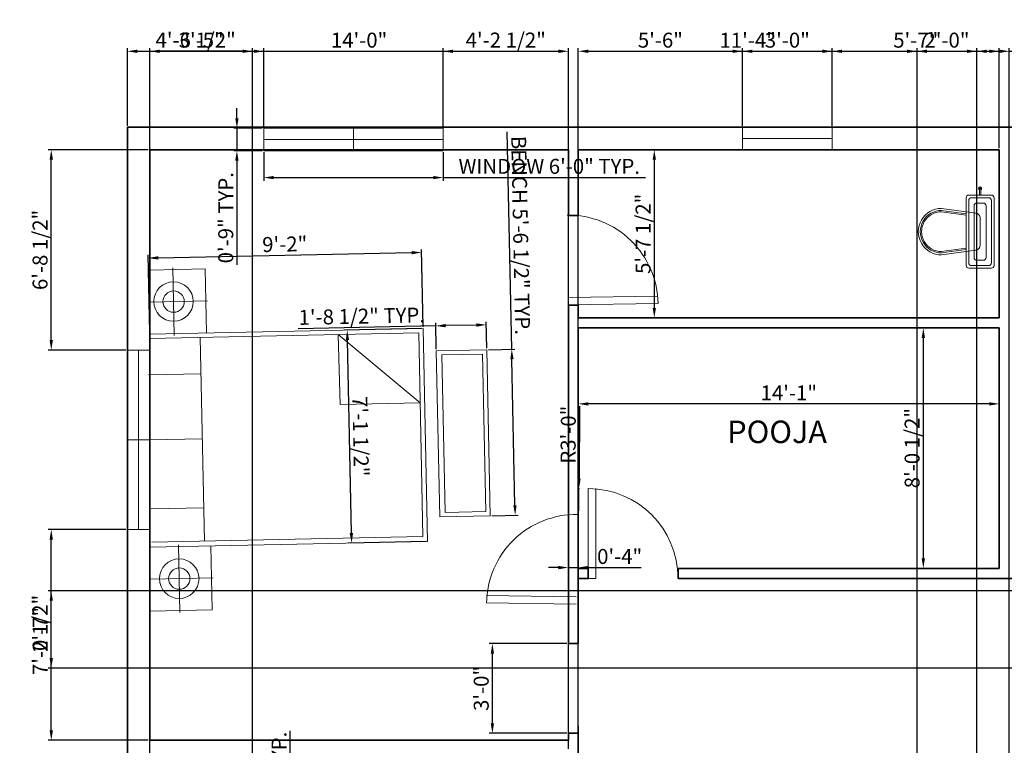
# Model space of a CAD drawing. Units: inches. Extents: x 1973 to 2661, y 1730 to 2412.
# Tile 3 of 5: x 1973 to 2368, y 2117 to 2409. Entities that reach past the tile are written whole.
import ezdxf

# ---------------------------------------------------------------- set-up
doc = ezdxf.new("R2010")
doc.units = ezdxf.units.IN
doc.linetypes.add('ACAD_ISO03W100', pattern=[30, 12, -18])
for name, color, linetype, lineweight in [('A-ANNO-DIMS', 2, 'Continuous', 18), ('A-AREA-IDEN', 7, 'Continuous', 25), ('A-DOOR', 3, 'Continuous', 18), ('A-FLOR-FIXT', 9, 'Continuous', 18), ('A-FLOR-FIXT-HIDN', 9, 'ACAD_ISO03W100', 13), ('A-FURN', 8, 'Continuous', 18), ('A-GLAZ', 4, 'Continuous', 18), ('A-WALL', 7, 'Continuous', 35)]:
    doc.layers.add(name, color=color, linetype=linetype, lineweight=lineweight)
doc.styles.get("Standard").update_dxf_attribs({"font": 'arial.ttf'})
doc.dimstyles.new('ISO-25', dxfattribs={"dimtxt": 6, "dimasz": 4, "dimexe": 1.25, "dimexo": 0.625, "dimtad": 1, "dimdec": 0, "dimrnd": 6, "dimlunit": 3, "dimtxsty": 'Standard', "dimcen": 2.5, "dimadec": 0, "dimazin": 0, "dimtfac": 1, "dimtdec": 0, "dimtmove": 0, "dimatfit": 3, "dimfxl": 1, "dimarcsym": 0})

# ---------------------------------------------------------------- blocks, each defined once
blk = doc.blocks.new('DOOR-36-SWING')
for p, q in [((0, 0), (0, 36)), ((0, 36), (0, 0)), ((3, 0), (3, 36)), ((0, 0), (3, 0))]:
    blk.add_line(p, q)
blk.add_arc((0, 0), 36, 0, 90)
blk = doc.blocks.new('WIN-72-TWO-LIGHT')
for p, q in [((0, 72), (9, 72)), ((0, 0), (0, 72)), ((4.5, 72), (4.5, 36)), ((9, 72), (9, 0)), ((4.5, 36), (0, 36)), ((0, 36), (9, 36)), ((4.5, 36), (4.5, 0)), ((9, 0), (0, 0))]:
    blk.add_line(p, q)
blk = doc.blocks.new('WC-TANK-PLAN')
for p, q in [((9.95, 11.2), (8.6, 21.07)), ((10.75, 11.2), (9.39, 21.19)), ((11.29, 11.2), (9.92, 21.26)), ((25.95, 21.26), (24.57, 11.2)), ((26.48, 21.19), (25.11, 11.2)), ((27.27, 21.07), (25.92, 11.2)), ((3.27, 1.07), (3.27, 10.13)), ((31.53, 11.2), (4.33, 11.2)), ((4.33, 2.13), (4.33, 9.07)), ((30.47, 10.13), (5.4, 10.13)), ((28.33, 8), (7.53, 8)), ((31.53, 2.13), (31.53, 9.07)), ((32.6, 1.07), (32.6, 10.13)), ((0.94, 5.6), (0.22, 5.6)), ((0.6, 5.33), (0.6, 5.87)), ((3.27, 5.87), (0.6, 5.87)), ((3.27, 5.33), (0.6, 5.33)), ((6.47, 4.27), (6.47, 6.93)), ((29.4, 4.27), (29.4, 6.93)), ((30.47, 1.07), (5.4, 1.07)), ((28.33, 3.2), (7.53, 3.2)), ((31.53, 0), (4.33, 0))]:
    blk.add_line(p, q)
for centre, radius, start, end in [((17.93, 21.07), 9.33, 0, 180), ((17.93, 21.07), 8.53, 0, 180), ((17.93, 21.07), 8, 0, 180), ((4.33, 10.13), 1.07, 90, 180), ((5.4, 9.07), 1.07, 90, 180), ((7.53, 6.93), 1.07, 90, 180), ((28.33, 6.93), 1.07, 0, 90), ((30.47, 9.07), 1.07, 0, 90), ((31.53, 10.13), 1.07, 0, 90), ((0.6, 5.6), 0.599, 26.4407, 333.5593), ((7.53, 4.27), 1.07, 180, 270), ((28.33, 4.27), 1.07, 270, 0), ((4.33, 1.07), 1.07, 180, 270), ((5.4, 2.13), 1.07, 180, 270), ((30.47, 2.13), 1.07, 270, 0), ((31.53, 1.07), 1.07, 270, 0)]:
    blk.add_arc(centre, radius, start, end)
blk = doc.blocks.new('BENCH-BED-END')
for p, q in [((0, 20.3), (0, 0)), ((66.64, 20.3), (0, 20.3)), ((66.64, 0), (66.64, 20.3)), ((1.73, 1.73), (1.73, 18.14)), ((1.73, 18.14), (64.92, 18.14)), ((64.92, 18.14), (64.92, 1.73)), ((64.92, 1.73), (1.73, 1.73)), ((0, 0), (66.64, 0))]:
    blk.add_line(p, q)
blk = doc.blocks.new('*D14')
at = {"layer": 'A-ANNO-DIMS', "color": 0, "lineweight": -2, "transparency": 16777216}
for p, q in [((2070.79, 2355.34), (2070.79, 2343.92)), ((2142.79, 2355.34), (2142.79, 2343.92)), ((2074.79, 2345.17), (2138.79, 2345.17)), ((2142.79, 2345.17), (2223.97, 2345.17))]:
    blk.add_line(p, q, dxfattribs=at)
at = {"layer": 'A-ANNO-DIMS', "color": 0, "transparency": 16777216}
for points in [[(2074.79, 2345.83), (2074.79, 2344.5), (2070.79, 2345.17)], [(2138.79, 2345.83), (2138.79, 2344.5), (2142.79, 2345.17)]]:
    blk.add_solid(points, dxfattribs=at)
at = {"layer": 'Defpoints', "color": 0, "transparency": 16777216}
for p in [(2070.79, 2355.97), (2142.79, 2355.97), (2142.79, 2345.17)]:
    blk.add_point(p, dxfattribs=at)
at = {"layer": 'A-ANNO-DIMS', "color": 0, "transparency": 16777216, "insert": (2185.38, 2348.9), "char_height": 6, "attachment_point": 5}
blk.add_mtext('WINDOW 6\'-0" TYP.', dxfattribs=at)
blk = doc.blocks.new('*D15')
at = {"layer": 'A-ANNO-DIMS', "color": 0, "lineweight": -2, "transparency": 16777216}
for p, q in [((2059.99, 2368.97), (2059.99, 2372.97)), ((2070.17, 2364.97), (2058.74, 2364.97)), ((2059.99, 2364.97), (2059.99, 2355.97)), ((2070.17, 2355.97), (2058.74, 2355.97)), ((2059.99, 2351.97), (2059.99, 2310.14))]:
    blk.add_line(p, q, dxfattribs=at)
at = {"layer": 'A-ANNO-DIMS', "color": 0, "transparency": 16777216}
for points in [[(2059.33, 2368.97), (2060.66, 2368.97), (2059.99, 2364.97)], [(2059.33, 2351.97), (2060.66, 2351.97), (2059.99, 2355.97)]]:
    blk.add_solid(points, dxfattribs=at)
at = {"layer": 'Defpoints', "color": 0, "transparency": 16777216}
for p in [(2070.79, 2364.97), (2059.99, 2355.97), (2070.79, 2355.97)]:
    blk.add_point(p, dxfattribs=at)
at = {"layer": 'A-ANNO-DIMS', "color": 0, "transparency": 16777216, "insert": (2056.3, 2329.06), "char_height": 6, "attachment_point": 5, "rotation": 90}
blk.add_mtext('0\'-9" TYP.', dxfattribs=at)
blk = doc.blocks.new('*D21')
at = {"layer": 'A-ANNO-DIMS', "color": 0, "lineweight": -2, "transparency": 16777216}
for p, q in [((2081.33, 2081.84), (2081.33, 2123.1)), ((2084.06, 2081.84), (2080.08, 2081.84)), ((2081.33, 2066.85), (2081.33, 2077.84)), ((2084.06, 2062.85), (2080.08, 2062.85))]:
    blk.add_line(p, q, dxfattribs=at)
at = {"layer": 'A-ANNO-DIMS', "color": 0, "transparency": 16777216}
for points in [[(2080.67, 2077.84), (2082, 2077.84), (2081.33, 2081.84)], [(2080.67, 2066.85), (2082, 2066.85), (2081.33, 2062.85)]]:
    blk.add_solid(points, dxfattribs=at)
at = {"layer": 'Defpoints', "color": 0, "transparency": 16777216}
for p in [(2081.33, 2081.84), (2084.68, 2081.84), (2084.68, 2062.85)]:
    blk.add_point(p, dxfattribs=at)
at = {"layer": 'A-ANNO-DIMS', "color": 0, "transparency": 16777216, "insert": (2077.7, 2104.47), "char_height": 6, "attachment_point": 5, "rotation": 90}
blk.add_mtext('1\'-7" TYP.', dxfattribs=at)
blk = doc.blocks.new('*D24')
at = {"layer": 'A-ANNO-DIMS', "color": 0, "lineweight": -2, "transparency": 16777216}
for p, q in [((2170.33, 2276.29), (2168.54, 2363.48)), ((2160.96, 2276.1), (2171.58, 2276.32)), ((2171.62, 2213.66), (2170.41, 2272.29)), ((2162.33, 2209.47), (2172.95, 2209.69))]:
    blk.add_line(p, q, dxfattribs=at)
at = {"layer": 'A-ANNO-DIMS', "color": 0, "transparency": 16777216}
for points in [[(2171.08, 2272.31), (2169.75, 2272.28), (2170.33, 2276.29)], [(2172.28, 2213.68), (2170.95, 2213.65), (2171.7, 2209.66)]]:
    blk.add_solid(points, dxfattribs=at)
at = {"layer": 'Defpoints', "color": 0, "transparency": 16777216}
for p in [(2160.34, 2276.09), (2170.33, 2276.29), (2161.7, 2209.46)]:
    blk.add_point(p, dxfattribs=at)
at = {"layer": 'A-ANNO-DIMS', "color": 0, "transparency": 16777216, "insert": (2173.12, 2321.96), "char_height": 6, "attachment_point": 5, "rotation": 271.1773}
blk.add_mtext('BENCH 5\'-6 1/2" TYP.', dxfattribs=at)
blk = doc.blocks.new('*D25')
at = {"layer": 'A-ANNO-DIMS', "color": 0, "lineweight": -2, "transparency": 16777216}
for p, q in [((2139.83, 2285.66), (2084.6, 2284.53)), ((2140.02, 2276.29), (2139.81, 2286.91)), ((2156.13, 2286), (2143.83, 2285.75)), ((2160.32, 2276.71), (2160.1, 2287.33))]:
    blk.add_line(p, q, dxfattribs=at)
at = {"layer": 'A-ANNO-DIMS', "color": 0, "transparency": 16777216}
for points in [[(2143.82, 2286.41), (2143.84, 2285.08), (2139.83, 2285.66)], [(2156.12, 2286.67), (2156.14, 2285.33), (2160.13, 2286.08)]]:
    blk.add_solid(points, dxfattribs=at)
at = {"layer": 'Defpoints', "color": 0, "transparency": 16777216}
for p in [(2139.83, 2285.66), (2140.04, 2275.67), (2160.34, 2276.09)]:
    blk.add_point(p, dxfattribs=at)
at = {"layer": 'A-ANNO-DIMS', "color": 0, "transparency": 16777216, "insert": (2110.14, 2288.78), "char_height": 6, "attachment_point": 5, "rotation": 1.1773}
blk.add_mtext('1\'-8 1/2" TYP.', dxfattribs=at)
blk = doc.blocks.new('*D32')
at = {"layer": 'A-ANNO-DIMS', "color": 0, "lineweight": -2, "transparency": 16777216}
for p, q in [((2016.04, 2365.98), (2016.04, 2397.1)), ((2020.04, 2395.85), (2066.79, 2395.85)), ((2070.79, 2365.59), (2070.79, 2397.1))]:
    blk.add_line(p, q, dxfattribs=at)
at = {"layer": 'A-ANNO-DIMS', "color": 0, "transparency": 16777216}
for points in [[(2020.04, 2396.52), (2020.04, 2395.18), (2016.04, 2395.85)], [(2066.79, 2396.52), (2066.79, 2395.18), (2070.79, 2395.85)]]:
    blk.add_solid(points, dxfattribs=at)
at = {"layer": 'Defpoints', "color": 0, "transparency": 16777216}
for p in [(2070.79, 2395.85), (2016.04, 2365.35), (2070.79, 2364.97)]:
    blk.add_point(p, dxfattribs=at)
at = {"layer": 'A-ANNO-DIMS', "color": 0, "transparency": 16777216, "insert": (2043.42, 2399.58), "char_height": 6, "attachment_point": 5}
blk.add_mtext('4\'-6 1/2"', dxfattribs=at)
blk = doc.blocks.new('*D33')
at = {"layer": 'A-ANNO-DIMS', "color": 0, "lineweight": -2, "transparency": 16777216}
for p, q in [((2142.79, 2365.59), (2142.79, 2397.1)), ((2146.79, 2395.85), (2189.04, 2395.85)), ((2193.04, 2356.98), (2193.04, 2397.1))]:
    blk.add_line(p, q, dxfattribs=at)
at = {"layer": 'A-ANNO-DIMS', "color": 0, "transparency": 16777216}
for points in [[(2146.79, 2396.52), (2146.79, 2395.18), (2142.79, 2395.85)], [(2189.04, 2396.52), (2189.04, 2395.18), (2193.04, 2395.85)]]:
    blk.add_solid(points, dxfattribs=at)
at = {"layer": 'Defpoints', "color": 0, "transparency": 16777216}
for p in [(2193.04, 2395.85), (2142.79, 2364.97), (2193.04, 2356.35)]:
    blk.add_point(p, dxfattribs=at)
at = {"layer": 'A-ANNO-DIMS', "color": 0, "transparency": 16777216, "insert": (2167.92, 2399.58), "char_height": 6, "attachment_point": 5}
blk.add_mtext('4\'-2 1/2"', dxfattribs=at)
blk = doc.blocks.new('*D34')
at = {"layer": 'A-ANNO-DIMS', "color": 0, "lineweight": -2, "transparency": 16777216}
for p, q in [((2197.04, 2356.98), (2197.04, 2397.1)), ((2201.04, 2395.85), (2258.95, 2395.85)), ((2262.95, 2365.95), (2262.95, 2397.1))]:
    blk.add_line(p, q, dxfattribs=at)
at = {"layer": 'A-ANNO-DIMS', "color": 0, "transparency": 16777216}
for points in [[(2201.04, 2396.52), (2201.04, 2395.18), (2197.04, 2395.85)], [(2258.95, 2396.52), (2258.95, 2395.18), (2262.95, 2395.85)]]:
    blk.add_solid(points, dxfattribs=at)
at = {"layer": 'Defpoints', "color": 0, "transparency": 16777216}
for p in [(2262.95, 2395.85), (2262.95, 2365.32), (2197.04, 2356.35)]:
    blk.add_point(p, dxfattribs=at)
at = {"layer": 'A-ANNO-DIMS', "color": 0, "transparency": 16777216, "insert": (2229.99, 2399.54), "char_height": 6, "attachment_point": 5}
blk.add_mtext('5\'-6"', dxfattribs=at)
blk = doc.blocks.new('*D35')
at = {"layer": 'A-ANNO-DIMS', "color": 0, "lineweight": -2, "transparency": 16777216}
for p, q in [((2262.95, 2365.95), (2262.95, 2397.1)), ((2266.95, 2395.85), (2294.95, 2395.85)), ((2298.95, 2365.95), (2298.95, 2397.1))]:
    blk.add_line(p, q, dxfattribs=at)
at = {"layer": 'A-ANNO-DIMS', "color": 0, "transparency": 16777216}
for points in [[(2266.95, 2396.52), (2266.95, 2395.18), (2262.95, 2395.85)], [(2294.95, 2396.52), (2294.95, 2395.18), (2298.95, 2395.85)]]:
    blk.add_solid(points, dxfattribs=at)
at = {"layer": 'Defpoints', "color": 0, "transparency": 16777216}
for p in [(2298.95, 2395.85), (2262.95, 2365.32), (2298.95, 2365.32)]:
    blk.add_point(p, dxfattribs=at)
at = {"layer": 'A-ANNO-DIMS', "color": 0, "transparency": 16777216, "insert": (2280.95, 2399.54), "char_height": 6, "attachment_point": 5}
blk.add_mtext('3\'-0"', dxfattribs=at)
blk = doc.blocks.new('*D36')
at = {"layer": 'A-ANNO-DIMS', "color": 0, "lineweight": -2, "transparency": 16777216}
for p, q in [((2298.95, 2365.95), (2298.95, 2397.1)), ((2302.95, 2395.85), (2362.04, 2395.85)), ((2366.04, 2356.98), (2366.04, 2397.1))]:
    blk.add_line(p, q, dxfattribs=at)
at = {"layer": 'A-ANNO-DIMS', "color": 0, "transparency": 16777216}
for points in [[(2302.95, 2396.52), (2302.95, 2395.18), (2298.95, 2395.85)], [(2362.04, 2396.52), (2362.04, 2395.18), (2366.04, 2395.85)]]:
    blk.add_solid(points, dxfattribs=at)
at = {"layer": 'Defpoints', "color": 0, "transparency": 16777216}
for p in [(2366.04, 2395.85), (2298.95, 2365.32), (2366.04, 2356.35)]:
    blk.add_point(p, dxfattribs=at)
at = {"layer": 'A-ANNO-DIMS', "color": 0, "transparency": 16777216, "insert": (2332.49, 2399.53), "char_height": 6, "attachment_point": 5}
blk.add_mtext('5\'-7"', dxfattribs=at)
blk = doc.blocks.new('*D44')
at = {"layer": 'A-ANNO-DIMS', "color": 0, "lineweight": -2, "transparency": 16777216}
for p, q in [((2015.35, 2203.93), (1984.22, 2203.93)), ((1985.47, 2123.35), (1985.47, 2199.93)), ((2024.42, 2119.35), (1984.22, 2119.35))]:
    blk.add_line(p, q, dxfattribs=at)
at = {"layer": 'A-ANNO-DIMS', "color": 0, "transparency": 16777216}
for points in [[(1984.81, 2199.93), (1986.14, 2199.93), (1985.47, 2203.93)], [(1984.81, 2123.35), (1986.14, 2123.35), (1985.47, 2119.35)]]:
    blk.add_solid(points, dxfattribs=at)
at = {"layer": 'Defpoints', "color": 0, "transparency": 16777216}
for p in [(1985.47, 2203.93), (2015.97, 2203.93), (2025.04, 2119.35)]:
    blk.add_point(p, dxfattribs=at)
at = {"layer": 'A-ANNO-DIMS', "color": 0, "transparency": 16777216, "insert": (1981.75, 2161.64), "char_height": 6, "attachment_point": 5, "rotation": 90}
blk.add_mtext('7\'-0 1/2"', dxfattribs=at)
blk = doc.blocks.new('*D45')
at = {"layer": 'A-ANNO-DIMS', "color": 0, "lineweight": -2, "transparency": 16777216}
for p, q in [((2024.42, 2356.35), (1984.22, 2356.35)), ((1985.47, 2279.93), (1985.47, 2352.35)), ((2015.35, 2275.93), (1984.22, 2275.93))]:
    blk.add_line(p, q, dxfattribs=at)
at = {"layer": 'A-ANNO-DIMS', "color": 0, "transparency": 16777216}
for points in [[(1984.81, 2352.35), (1986.14, 2352.35), (1985.47, 2356.35)], [(1984.81, 2279.93), (1986.14, 2279.93), (1985.47, 2275.93)]]:
    blk.add_solid(points, dxfattribs=at)
at = {"layer": 'Defpoints', "color": 0, "transparency": 16777216}
for p in [(1985.47, 2356.35), (2025.04, 2356.35), (2015.97, 2275.93)]:
    blk.add_point(p, dxfattribs=at)
at = {"layer": 'A-ANNO-DIMS', "color": 0, "transparency": 16777216, "insert": (1981.75, 2316.14), "char_height": 6, "attachment_point": 5, "rotation": 90}
blk.add_mtext('6\'-8 1/2"', dxfattribs=at)
blk = doc.blocks.new('*D46')
at = {"layer": 'A-ANNO-DIMS', "color": 0, "lineweight": -2, "transparency": 16777216}
for p, q in [((2025.04, 2115.98), (2025.04, 2397.1)), ((2029.04, 2395.85), (2189.04, 2395.85)), ((2193.04, 2115.98), (2193.04, 2397.1))]:
    blk.add_line(p, q, dxfattribs=at)
at = {"layer": 'A-ANNO-DIMS', "color": 0, "transparency": 16777216}
for points in [[(2029.04, 2396.52), (2029.04, 2395.18), (2025.04, 2395.85)], [(2189.04, 2396.52), (2189.04, 2395.18), (2193.04, 2395.85)]]:
    blk.add_solid(points, dxfattribs=at)
at = {"layer": 'Defpoints', "color": 0, "transparency": 16777216}
for p in [(2193.04, 2395.85), (2025.04, 2115.35), (2193.04, 2115.35)]:
    blk.add_point(p, dxfattribs=at)
at = {"layer": 'A-ANNO-DIMS', "color": 0, "transparency": 16777216, "insert": (2109.04, 2399.54), "char_height": 6, "attachment_point": 5}
blk.add_mtext('14\'-0"', dxfattribs=at)
blk = doc.blocks.new('*D47')
at = {"layer": 'A-ANNO-DIMS', "color": 0, "lineweight": -2, "transparency": 16777216}
for p, q in [((2197.67, 2356.35), (2228.79, 2356.35)), ((2227.54, 2352.35), (2227.54, 2292.85)), ((2197.67, 2288.85), (2228.79, 2288.85))]:
    blk.add_line(p, q, dxfattribs=at)
at = {"layer": 'A-ANNO-DIMS', "color": 0, "transparency": 16777216}
for points in [[(2226.88, 2352.35), (2228.21, 2352.35), (2227.54, 2356.35)], [(2226.88, 2292.85), (2228.21, 2292.85), (2227.54, 2288.85)]]:
    blk.add_solid(points, dxfattribs=at)
at = {"layer": 'Defpoints', "color": 0, "transparency": 16777216}
for p in [(2197.04, 2356.35), (2197.04, 2288.85), (2227.54, 2288.85)]:
    blk.add_point(p, dxfattribs=at)
at = {"layer": 'A-ANNO-DIMS', "color": 0, "transparency": 16777216, "insert": (2223.81, 2322.6), "char_height": 6, "attachment_point": 5, "rotation": 90}
blk.add_mtext('5\'-7 1/2"', dxfattribs=at)
blk = doc.blocks.new('*D48')
at = {"layer": 'A-ANNO-DIMS', "color": 0, "lineweight": -2, "transparency": 16777216}
for p, q in [((2365.42, 2284.85), (2334.29, 2284.85)), ((2335.54, 2192.35), (2335.54, 2280.85)), ((2365.42, 2188.35), (2334.29, 2188.35))]:
    blk.add_line(p, q, dxfattribs=at)
at = {"layer": 'A-ANNO-DIMS', "color": 0, "transparency": 16777216}
for points in [[(2334.88, 2280.85), (2336.21, 2280.85), (2335.54, 2284.85)], [(2334.88, 2192.35), (2336.21, 2192.35), (2335.54, 2188.35)]]:
    blk.add_solid(points, dxfattribs=at)
at = {"layer": 'Defpoints', "color": 0, "transparency": 16777216}
for p in [(2335.54, 2284.85), (2366.04, 2284.85), (2366.04, 2188.35)]:
    blk.add_point(p, dxfattribs=at)
at = {"layer": 'A-ANNO-DIMS', "color": 0, "transparency": 16777216, "insert": (2331.81, 2236.6), "char_height": 6, "attachment_point": 5, "rotation": 90}
blk.add_mtext('8\'-0 1/2"', dxfattribs=at)
blk = doc.blocks.new('*D49')
at = {"layer": 'A-ANNO-DIMS', "color": 0, "lineweight": -2, "transparency": 16777216}
for p, q in [((2197.04, 2284.23), (2197.04, 2253.1)), ((2366.04, 2284.23), (2366.04, 2253.1)), ((2362.04, 2254.35), (2201.04, 2254.35))]:
    blk.add_line(p, q, dxfattribs=at)
at = {"layer": 'A-ANNO-DIMS', "color": 0, "transparency": 16777216}
for points in [[(2201.04, 2255.02), (2201.04, 2253.68), (2197.04, 2254.35)], [(2362.04, 2255.02), (2362.04, 2253.68), (2366.04, 2254.35)]]:
    blk.add_solid(points, dxfattribs=at)
at = {"layer": 'Defpoints', "color": 0, "transparency": 16777216}
for p in [(2197.04, 2284.85), (2366.04, 2284.85), (2197.04, 2254.35)]:
    blk.add_point(p, dxfattribs=at)
at = {"layer": 'A-ANNO-DIMS', "color": 0, "transparency": 16777216, "insert": (2281.54, 2257.99), "char_height": 6, "attachment_point": 5}
blk.add_mtext('14\'-1"', dxfattribs=at)
blk = doc.blocks.new('*D54')
at = {"layer": 'A-ANNO-DIMS', "color": 0, "lineweight": -2, "transparency": 16777216}
for p, q in [((2197.04, 1834.98), (2197.04, 2397.1)), ((2201.04, 2395.85), (2329.03, 2395.85)), ((2333.03, 1834.87), (2333.03, 2397.1))]:
    blk.add_line(p, q, dxfattribs=at)
at = {"layer": 'A-ANNO-DIMS', "color": 0, "transparency": 16777216}
for points in [[(2201.04, 2396.52), (2201.04, 2395.18), (2197.04, 2395.85)], [(2329.03, 2396.52), (2329.03, 2395.18), (2333.03, 2395.85)]]:
    blk.add_solid(points, dxfattribs=at)
at = {"layer": 'Defpoints', "color": 0, "transparency": 16777216}
for p in [(2333.03, 2395.85), (2197.04, 1834.35), (2333.03, 1834.25)]:
    blk.add_point(p, dxfattribs=at)
at = {"layer": 'A-ANNO-DIMS', "color": 0, "transparency": 16777216, "insert": (2265.03, 2399.49), "char_height": 6, "attachment_point": 5}
blk.add_mtext('11\'-4"', dxfattribs=at)
blk = doc.blocks.new('*D61')
at = {"layer": 'A-ANNO-DIMS', "color": 0, "lineweight": -2, "transparency": 16777216}
for p, q in [((2606.42, 2179.35), (1984.22, 2179.35)), ((1985.47, 2152.35), (1985.47, 2175.35)), ((2606.42, 2148.35), (1984.22, 2148.35))]:
    blk.add_line(p, q, dxfattribs=at)
at = {"layer": 'A-ANNO-DIMS', "color": 0, "transparency": 16777216}
for points in [[(1984.81, 2175.35), (1986.14, 2175.35), (1985.47, 2179.35)], [(1984.81, 2152.35), (1986.14, 2152.35), (1985.47, 2148.35)]]:
    blk.add_solid(points, dxfattribs=at)
at = {"layer": 'Defpoints', "color": 0, "transparency": 16777216}
for p in [(1985.47, 2179.35), (2607.04, 2179.35), (2607.04, 2148.35)]:
    blk.add_point(p, dxfattribs=at)
at = {"layer": 'A-ANNO-DIMS', "color": 0, "transparency": 16777216, "insert": (1981.84, 2163.85), "char_height": 6, "attachment_point": 5, "rotation": 90}
blk.add_mtext('2\'-7"', dxfattribs=at)
blk = doc.blocks.new('*D66')
at = {"layer": 'A-ANNO-DIMS', "color": 0, "lineweight": -2, "transparency": 16777216}
for p, q in [((2333.03, 1843.98), (2333.03, 2397.1)), ((2337.03, 2395.85), (2353.02, 2395.85)), ((2357.02, 1843.98), (2357.02, 2397.1))]:
    blk.add_line(p, q, dxfattribs=at)
at = {"layer": 'A-ANNO-DIMS', "color": 0, "transparency": 16777216}
for points in [[(2337.03, 2396.52), (2337.03, 2395.18), (2333.03, 2395.85)], [(2353.02, 2396.52), (2353.02, 2395.18), (2357.02, 2395.85)]]:
    blk.add_solid(points, dxfattribs=at)
at = {"layer": 'Defpoints', "color": 0, "transparency": 16777216}
for p in [(2357.02, 2395.85), (2333.03, 1843.35), (2357.02, 1843.35)]:
    blk.add_point(p, dxfattribs=at)
at = {"layer": 'A-ANNO-DIMS', "color": 0, "transparency": 16777216, "insert": (2345.02, 2399.54), "char_height": 6, "attachment_point": 5}
blk.add_mtext('2\'-0"', dxfattribs=at)
blk = doc.blocks.new('*D69')
at = {"layer": 'A-ANNO-DIMS', "color": 0, "lineweight": -2, "transparency": 16777216}
for p, q in [((2357.02, 1843.98), (2357.02, 2397.1)), ((2361.02, 2395.85), (2366.04, 2395.85)), ((2370.04, 1843.98), (2370.04, 2397.1)), ((2370.04, 2395.85), (2390.68, 2395.85))]:
    blk.add_line(p, q, dxfattribs=at)
at = {"layer": 'A-ANNO-DIMS', "color": 0, "transparency": 16777216}
for points in [[(2361.02, 2396.52), (2361.02, 2395.18), (2357.02, 2395.85)], [(2366.04, 2396.52), (2366.04, 2395.18), (2370.04, 2395.85)]]:
    blk.add_solid(points, dxfattribs=at)
at = {"layer": 'Defpoints', "color": 0, "transparency": 16777216}
for p in [(2370.04, 2395.85), (2357.02, 1843.35), (2370.04, 1843.35)]:
    blk.add_point(p, dxfattribs=at)
at = {"layer": 'A-ANNO-DIMS', "color": 0, "transparency": 16777216, "insert": (2382.36, 2399.49), "char_height": 6, "attachment_point": 5}
blk.add_mtext('1\'-1"', dxfattribs=at)
blk = doc.blocks.new('*D72')
at = {"layer": 'A-ANNO-DIMS', "color": 0, "lineweight": -2, "transparency": 16777216}
for p, q in [((2025.04, 1930.6), (2025.04, 2397.1)), ((2062.26, 2395.85), (2029.04, 2395.85)), ((2066.26, 1930.6), (2066.26, 2397.1))]:
    blk.add_line(p, q, dxfattribs=at)
at = {"layer": 'A-ANNO-DIMS', "color": 0, "transparency": 16777216}
for points in [[(2029.04, 2396.52), (2029.04, 2395.18), (2025.04, 2395.85)], [(2062.26, 2396.52), (2062.26, 2395.18), (2066.26, 2395.85)]]:
    blk.add_solid(points, dxfattribs=at)
at = {"layer": 'Defpoints', "color": 0, "transparency": 16777216}
for p in [(2025.04, 2395.85), (2025.04, 1929.97), (2066.26, 1929.97)]:
    blk.add_point(p, dxfattribs=at)
at = {"layer": 'A-ANNO-DIMS', "color": 0, "transparency": 16777216, "insert": (2045.65, 2399.54), "char_height": 6, "attachment_point": 5}
blk.add_mtext('3\'-5"', dxfattribs=at)
blk = doc.blocks.new('*D76')
at = {"layer": 'A-ANNO-DIMS', "color": 0, "lineweight": -2, "transparency": 16777216}
for p, q in [((2192.42, 2158.17), (2161.29, 2158.17)), ((2162.54, 2126.17), (2162.54, 2154.17)), ((2192.42, 2122.17), (2161.29, 2122.17))]:
    blk.add_line(p, q, dxfattribs=at)
at = {"layer": 'A-ANNO-DIMS', "color": 0, "transparency": 16777216}
for points in [[(2161.88, 2154.17), (2163.21, 2154.17), (2162.54, 2158.17)], [(2161.88, 2126.17), (2163.21, 2126.17), (2162.54, 2122.17)]]:
    blk.add_solid(points, dxfattribs=at)
at = {"layer": 'Defpoints', "color": 0, "transparency": 16777216}
for p in [(2162.54, 2158.17), (2193.04, 2158.17), (2193.04, 2122.17)]:
    blk.add_point(p, dxfattribs=at)
at = {"layer": 'A-ANNO-DIMS', "color": 0, "transparency": 16777216, "insert": (2158.85, 2140.17), "char_height": 6, "attachment_point": 5, "rotation": 90}
blk.add_mtext('3\'-0"', dxfattribs=at)
blk = doc.blocks.new('*D77')
at = {"layer": 'A-ANNO-DIMS', "color": 0, "lineweight": -2, "transparency": 16777216}
for p, q in [((2193.04, 2158.79), (2193.04, 2189.92)), ((2197.04, 2158.79), (2197.04, 2189.92)), ((2189.04, 2188.67), (2185.04, 2188.67)), ((2193.04, 2188.67), (2197.04, 2188.67)), ((2201.04, 2188.67), (2222.24, 2188.67))]:
    blk.add_line(p, q, dxfattribs=at)
at = {"layer": 'A-ANNO-DIMS', "color": 0, "transparency": 16777216}
for points in [[(2189.04, 2189.34), (2189.04, 2188), (2193.04, 2188.67)], [(2201.04, 2189.34), (2201.04, 2188), (2197.04, 2188.67)]]:
    blk.add_solid(points, dxfattribs=at)
at = {"layer": 'Defpoints', "color": 0, "transparency": 16777216}
for p in [(2197.04, 2188.67), (2193.04, 2158.17), (2197.04, 2158.17)]:
    blk.add_point(p, dxfattribs=at)
at = {"layer": 'A-ANNO-DIMS', "color": 0, "transparency": 16777216, "insert": (2213.64, 2192.36), "char_height": 6, "attachment_point": 5}
blk.add_mtext('0\'-4"', dxfattribs=at)
blk = doc.blocks.new('*D80')
at = {"layer": 'A-ANNO-DIMS', "color": 0, "lineweight": -2, "transparency": 16777216}
for p, q in [((2134.76, 2285.25), (2134.12, 2316.37)), ((2025.03, 2283), (2024.39, 2314.12)), ((2028.41, 2312.95), (2130.15, 2315.04))]:
    blk.add_line(p, q, dxfattribs=at)
at = {"layer": 'A-ANNO-DIMS', "color": 0, "transparency": 16777216}
for points in [[(2028.4, 2313.61), (2028.43, 2312.28), (2024.42, 2312.87)], [(2130.14, 2315.71), (2130.17, 2314.37), (2134.15, 2315.12)]]:
    blk.add_solid(points, dxfattribs=at)
at = {"layer": 'Defpoints', "color": 0, "transparency": 16777216}
for p in [(2134.15, 2315.12), (2134.78, 2284.63), (2025.04, 2282.37)]:
    blk.add_point(p, dxfattribs=at)
at = {"layer": 'A-ANNO-DIMS', "color": 0, "transparency": 16777216, "insert": (2079.21, 2317.68), "char_height": 6, "attachment_point": 5, "rotation": 1.1773}
blk.add_mtext('9\'-2"', dxfattribs=at)
blk = doc.blocks.new('*D81')
at = {"layer": 'A-ANNO-DIMS', "color": 0, "lineweight": -2, "transparency": 16777216}
for p, q in [((2134.15, 2284.61), (2103.03, 2283.97)), ((2105.96, 2202.49), (2104.37, 2280)), ((2135.91, 2199.11), (2104.79, 2198.47))]:
    blk.add_line(p, q, dxfattribs=at)
at = {"layer": 'A-ANNO-DIMS', "color": 0, "transparency": 16777216}
for points in [[(2105.03, 2280.01), (2103.7, 2279.99), (2104.28, 2284)], [(2106.63, 2202.51), (2105.29, 2202.48), (2106.04, 2198.49)]]:
    blk.add_solid(points, dxfattribs=at)
at = {"layer": 'Defpoints', "color": 0, "transparency": 16777216}
for p in [(2134.78, 2284.63), (2104.28, 2284), (2136.53, 2199.12)]:
    blk.add_point(p, dxfattribs=at)
at = {"layer": 'A-ANNO-DIMS', "color": 0, "transparency": 16777216, "insert": (2108.89, 2241.32), "char_height": 6, "attachment_point": 5, "rotation": 271.1773}
blk.add_mtext('7\'-1 1/2"', dxfattribs=at)
blk = doc.blocks.new('*D83')
at = {"layer": 'A-ANNO-DIMS', "color": 0, "lineweight": -2, "transparency": 16777216}
for p, q in [((2197.54, 2253.42), (2197.33, 2224.35)), ((2197.04, 2184.35), (2197.3, 2220.35))]:
    blk.add_line(p, q, dxfattribs=at)
at = {"layer": 'A-ANNO-DIMS', "color": 0, "transparency": 16777216}
blk.add_solid([(2196.67, 2224.36), (2198, 2224.35), (2197.3, 2220.35)], dxfattribs=at)
at = {"layer": 'Defpoints', "color": 0, "transparency": 16777216}
for p in [(2197.3, 2220.35), (2197.04, 2184.35)]:
    blk.add_point(p, dxfattribs=at)
at = {"layer": 'A-ANNO-DIMS', "color": 0, "transparency": 16777216, "insert": (2193.77, 2241.98), "char_height": 6, "attachment_point": 5, "rotation": 89.5833}
blk.add_mtext('R3\'-0"', dxfattribs=at)

msp = doc.modelspace()

# ---------------------------------------------------------------- linework, layer by layer
at = {"layer": 'A-DOOR'}
for p, q in [((2197.04, 2187.35), (2197.09, 2187.35)), ((2197.09, 2187.35), (2197.04, 2187.35)), ((2197.09, 2187.35), (2197.04, 2187.35)), ((2197.04, 2187.35), (2197.09, 2187.35)), ((2160.2, 2174.49), (2196.19, 2173.97)), ((2196.19, 2173.97), (2160.2, 2174.49)), ((2160.24, 2177.49), (2196.23, 2176.97))]:
    msp.add_line(p, q, dxfattribs=at)
for centre, end in [((2197.04, 2184.35), 90), ((2197.04, 2184.35), 90), ((2197.04, 2184.35), 90), ((2197.04, 2184.35), 90), ((2196.19, 2173.97), 179.1676)]:
    msp.add_arc(centre, 36, 89.1676, end, dxfattribs=at)
at = {"layer": 'A-FLOR-FIXT-HIDN'}
msp.add_lwpolyline([(2352.72, 2331.46), (2356.5, 2330.95, -0.371763), (2358.32, 2328.83), (2358.32, 2318.12, -0.371763), (2356.5, 2316), (2352.72, 2315.49)], format="xyb", dxfattribs=at)
at = {"layer": 'A-FURN'}
for p, q in [((2025.04, 2308.04), (2047.26, 2308.49)), ((2034.85, 2281.85, -15.39), (2034.29, 2308.99, -15.39)), ((2047.26, 2308.49), (2047.79, 2282.84)), ((2025.04, 2295.22, -15.39), (2048.14, 2295.7, -15.39)), ((2134.78, 2284.63), (2025.04, 2282.37)), ((2136.53, 2199.12), (2134.78, 2284.63)), ((2132.98, 2282.86), (2025.04, 2280.65)), ((2046.98, 2199.33), (2045.3, 2281.06)), ((2101.49, 2254.15), (2100.58, 2282.2)), ((2100.58, 2282.2), (2133.55, 2254.81)), ((2134.66, 2201.13), (2132.98, 2282.86)), ((2024.44, 2265.95), (2045.6, 2266.39)), ((2133.55, 2254.81), (2101.49, 2254.15)), ((2024.97, 2239.93), (2046.14, 2240.37)), ((2024.99, 2228.83), (2025.04, 2226.21)), ((2025.54, 2212.27), (2046.71, 2212.71)), ((2025.04, 2196.83), (2136.53, 2199.12)), ((2025.82, 2198.89), (2134.66, 2201.13)), ((2037.13, 2170.65, -15.39), (2036.57, 2197.79, -15.39)), ((2050.07, 2171.68), (2049.54, 2197.33)), ((2025.04, 2183.98, -15.39), (2050.42, 2184.5, -15.39)), ((2025.04, 2171.16), (2050.07, 2171.68))]:
    msp.add_line(p, q, dxfattribs=at)
for centre, radius in [((2034.57, 2295.42, -15.39), 7.93), ((2034.57, 2295.42, -15.39), 4.28), ((2036.85, 2184.22, -15.39), 7.93), ((2036.85, 2184.22, -15.39), 4.28)]:
    msp.add_circle(centre, radius, dxfattribs=at)
at = {"layer": 'A-GLAZ'}
for p, q in [((2262.95, 2365.32), (2298.95, 2365.32)), ((2262.95, 2356.32), (2262.95, 2365.32)), ((2262.95, 2365.32), (2262.95, 2360.82)), ((2279.57, 2365.32), (2298.95, 2365.32)), ((2298.95, 2365.32), (2298.95, 2356.32)), ((2262.95, 2360.82), (2298.95, 2360.82)), ((2298.95, 2360.82), (2279.57, 2360.82)), ((2298.95, 2356.32), (2262.95, 2356.32)), ((2279.57, 2356.35), (2279.57, 2356.32)), ((2279.57, 2356.32), (2298.95, 2356.32))]:
    msp.add_line(p, q, dxfattribs=at)
at = {"layer": 'A-WALL'}
for p, q in [((2016.04, 1765.35), (2016.04, 2365.35)), ((2016.04, 2365.35), (2616.04, 2365.35)), ((2025.04, 2119.35), (2025.04, 2356.35)), ((2025.04, 2356.35), (2193.04, 2356.35)), ((2193.04, 2356.35), (2193.04, 2329.91)), ((2193.04, 2329.91), (2193.04, 2356.35)), ((2197.04, 2329.91), (2197.04, 2356.35)), ((2197.04, 2356.35), (2366.04, 2356.35)), ((2366.04, 2356.35), (2366.04, 2288.85)), ((2193.04, 2329.91), (2197.04, 2329.91)), ((2197.04, 2293.91), (2193.04, 2293.91)), ((2193.04, 2293.91), (2193.04, 2158.17)), ((2197.04, 2288.85), (2197.04, 2293.91)), ((2366.04, 2288.85), (2197.04, 2288.85)), ((2197.04, 2188.35), (2197.04, 2284.85)), ((2197.04, 2284.85), (2366.04, 2284.85)), ((2366.04, 2284.85), (2366.04, 2188.35)), ((2197.04, 2184.35), (2197.04, 2188.35)), ((2197.04, 2188.35), (2201.06, 2188.35)), ((2197.04, 2187.35), (2197.04, 2184.35)), ((2197.04, 2184.35), (2197.04, 2187.35)), ((2197.04, 2187.35), (2197.04, 2184.35)), ((2201.06, 2188.35), (2201.06, 2184.35)), ((2366.04, 2188.35), (2237.06, 2188.35)), ((2237.06, 2188.35), (2237.06, 2184.35)), ((2197.04, 2158.17), (2197.04, 2184.35)), ((2197.04, 2184.35), (2201.06, 2184.35)), ((2201.06, 2184.35), (2197.04, 2184.35)), ((2237.06, 2184.35), (2375.94, 2184.35)), ((2193.04, 2158.17), (2197.04, 2158.17)), ((2197.04, 2112.1), (2197.04, 2125.17)), ((2197.04, 2125.17), (2197.04, 2122.17)), ((2193.04, 2119.35), (2025.04, 2119.35)), ((2193.04, 2122.23), (2193.04, 2119.35)), ((2197.04, 2122.17), (2193.04, 2122.17)), ((2193.04, 2122.17), (2193.04, 2119.35))]:
    msp.add_line(p, q, dxfattribs=at)

# ---------------------------------------------------------------- block references
at = {"layer": 'A-DOOR', "extrusion": (0, 0, -1), "zscale": -1, "rotation": 89.16759712053707}
msp.add_blockref('DOOR-36-SWING', (-2193.07, 2294.09), dxfattribs=at)
at = {"layer": 'A-DOOR'}
msp.add_blockref('DOOR-36-SWING', (2201.06, 2184.35), dxfattribs=at)
at = {"layer": 'A-FLOR-FIXT', "extrusion": (0, 0, -1), "zscale": -1, "rotation": 269.999999999998}
msp.add_blockref('WC-TANK-PLAN', (-2363.92, 2341.41), dxfattribs=at)
at = {"layer": 'A-FURN', "rotation": 91.17731989174982}
msp.add_blockref('BENCH-BED-END', (2161.7, 2209.46), dxfattribs=at)
at = {"layer": 'A-GLAZ', "rotation": 269.9999999999997}
msp.add_blockref('WIN-72-TWO-LIGHT', (2070.79, 2364.97), dxfattribs=at)
at = {"layer": 'A-GLAZ'}
msp.add_blockref('WIN-72-TWO-LIGHT', (2015.97, 2203.93), dxfattribs=at)

# ---------------------------------------------------------------- texts
at = {"layer": 'A-AREA-IDEN', "insert": (2256.83, 2247.64), "char_height": 9, "attachment_point": 1}
msp.add_mtext_dynamic_manual_height_columns('POOJA', width=6.3229, gutter_width=12.5, heights=[0], dxfattribs=at)

# ---------------------------------------------------------------- dimensions: what is measured, and where the dimension line sits
at = {"layer": 'A-ANNO-DIMS'}
for base, p1, p2, picture, middle in [((2070.792, 2395.8513), (2016.0422, 2365.3513), (2070.792, 2364.9675), '*D32', (2043.4171, 2399.5786)), ((2193.0422, 2395.8513), (2142.792, 2364.9675), (2193.0422, 2356.3513), '*D33', (2167.9171, 2399.5786)), ((2193.04, 2395.85), (2025.04, 2115.35), (2193.04, 2115.35), '*D46', (2109.04, 2399.54)), ((2025.04, 2395.85), (2066.26, 1929.97), (2025.04, 1929.97), '*D72', (2045.65, 2399.54)), ((2262.95, 2395.85), (2197.04, 2356.35), (2262.95, 2365.32), '*D34', (2229.99, 2399.54)), ((2333.03, 2395.85), (2197.04, 1834.35), (2333.03, 1834.25), '*D54', (2265.03, 2399.49)), ((2298.95, 2395.85), (2262.95, 2365.32), (2298.95, 2365.32), '*D35', (2280.95, 2399.54)), ((2366.04, 2395.85), (2298.95, 2365.32), (2366.04, 2356.35), '*D36', (2332.49, 2399.53)), ((2357.02, 2395.85), (2333.03, 1843.35), (2357.02, 1843.35), '*D66', (2345.02, 2399.54)), ((2370.04, 2395.85), (2357.02, 1843.35), (2370.04, 1843.35), '*D69', (2382.36, 2399.49)), ((2197.04, 2188.67), (2193.04, 2158.17), (2197.04, 2158.17), '*D77', (2213.64, 2192.36))]:
    dim = msp.add_linear_dim(base=base, p1=p1, p2=p2, dimstyle='ISO-25', override={"dimdec": 1, "dimlfac": 1, "dimrnd": 0, "dimzin": 1, "dimdsep": 46, "dimlunit": 4, "dimfrac": 2}, dxfattribs=at)
    dim.commit()
    dim.dimension.update_dxf_attribs({"geometry": picture, "text_midpoint": middle})
for base, p1, p2, angle, text, picture, middle in [((2059.99, 2355.97), (2070.79, 2364.97), (2070.79, 2355.97), 270, '<> TYP.', '*D15', (2056.3, 2329.06)), ((2170.33, 2276.29), (2161.7, 2209.46), (2160.34, 2276.09), 91.1773, 'BENCH <> TYP.', '*D24', (2173.12, 2321.96)), ((2139.83, 2285.66), (2160.34, 2276.09), (2140.04, 2275.67), 181.1773, '<> TYP.', '*D25', (2110.14, 2288.78)), ((2081.33, 2081.84), (2084.68, 2062.85), (2084.68, 2081.84), 90, '<> TYP.', '*D21', (2077.7, 2104.47))]:
    dim = msp.add_linear_dim(base=base, p1=p1, p2=p2, angle=angle, text=text, dimstyle='ISO-25', override={"dimdec": 1, "dimlfac": 1, "dimrnd": 0, "dimzin": 1, "dimdsep": 46, "dimlunit": 4, "dimfrac": 2}, dxfattribs=at)
    dim.commit()
    dim.dimension.update_dxf_attribs({"geometry": picture, "text_midpoint": middle})
dim = msp.add_linear_dim(base=(2142.79, 2345.17), p1=(2070.79, 2355.97), p2=(2142.79, 2355.97), text='WINDOW <> TYP.', dimstyle='ISO-25', override={"dimdec": 1, "dimlfac": 1, "dimrnd": 0, "dimzin": 1, "dimdsep": 46, "dimlunit": 4, "dimfrac": 2}, dxfattribs=at)
dim.commit()
dim.dimension.update_dxf_attribs({"geometry": '*D14', "text_midpoint": (2185.38, 2348.9)})
for base, p1, p2, angle, picture, middle in [((1985.47, 2356.35), (2015.97, 2275.93), (2025.04, 2356.35), 90, '*D45', (1981.75, 2316.14)), ((2227.54, 2288.85), (2197.04, 2356.35), (2197.04, 2288.85), 270, '*D47', (2223.81, 2322.6)), ((2134.15, 2315.12), (2025.04, 2282.37), (2134.78, 2284.63), 1.1773, '*D80', (2079.21, 2317.68)), ((2104.28, 2284), (2136.53, 2199.12), (2134.78, 2284.63), 91.1773, '*D81', (2108.89, 2241.32)), ((2197.04, 2254.35), (2366.04, 2284.85), (2197.04, 2284.85), 180, '*D49', (2281.54, 2257.99)), ((2335.54, 2284.85), (2366.04, 2188.35), (2366.04, 2284.85), 90, '*D48', (2331.81, 2236.6)), ((1985.47, 2203.93), (2025.04, 2119.35), (2015.97, 2203.93), 90, '*D44', (1981.75, 2161.64)), ((1985.47, 2179.35), (2607.04, 2148.35), (2607.04, 2179.35), 90, '*D61', (1981.84, 2163.85)), ((2162.54, 2158.17), (2193.04, 2122.17), (2193.04, 2158.17), 90, '*D76', (2158.85, 2140.17))]:
    dim = msp.add_linear_dim(base=base, p1=p1, p2=p2, angle=angle, dimstyle='ISO-25', override={"dimdec": 1, "dimlfac": 1, "dimrnd": 0, "dimzin": 1, "dimdsep": 46, "dimlunit": 4, "dimfrac": 2}, dxfattribs=at)
    dim.commit()
    dim.dimension.update_dxf_attribs({"geometry": picture, "text_midpoint": middle})
dim = msp.add_radius_dim(center=(2197.04, 2184.35), mpoint=(2197.3, 2220.35), dimstyle='ISO-25', override={"dimdec": 1, "dimlfac": 1, "dimrnd": 0, "dimzin": 1, "dimdsep": 46, "dimlunit": 4, "dimfrac": 2}, dxfattribs=at)
dim.commit()
dim.dimension.update_dxf_attribs({"geometry": '*D83', "text_midpoint": (2197.46, 2241.95), "dimtype": 164})

doc.saveas('drawing.dxf')
